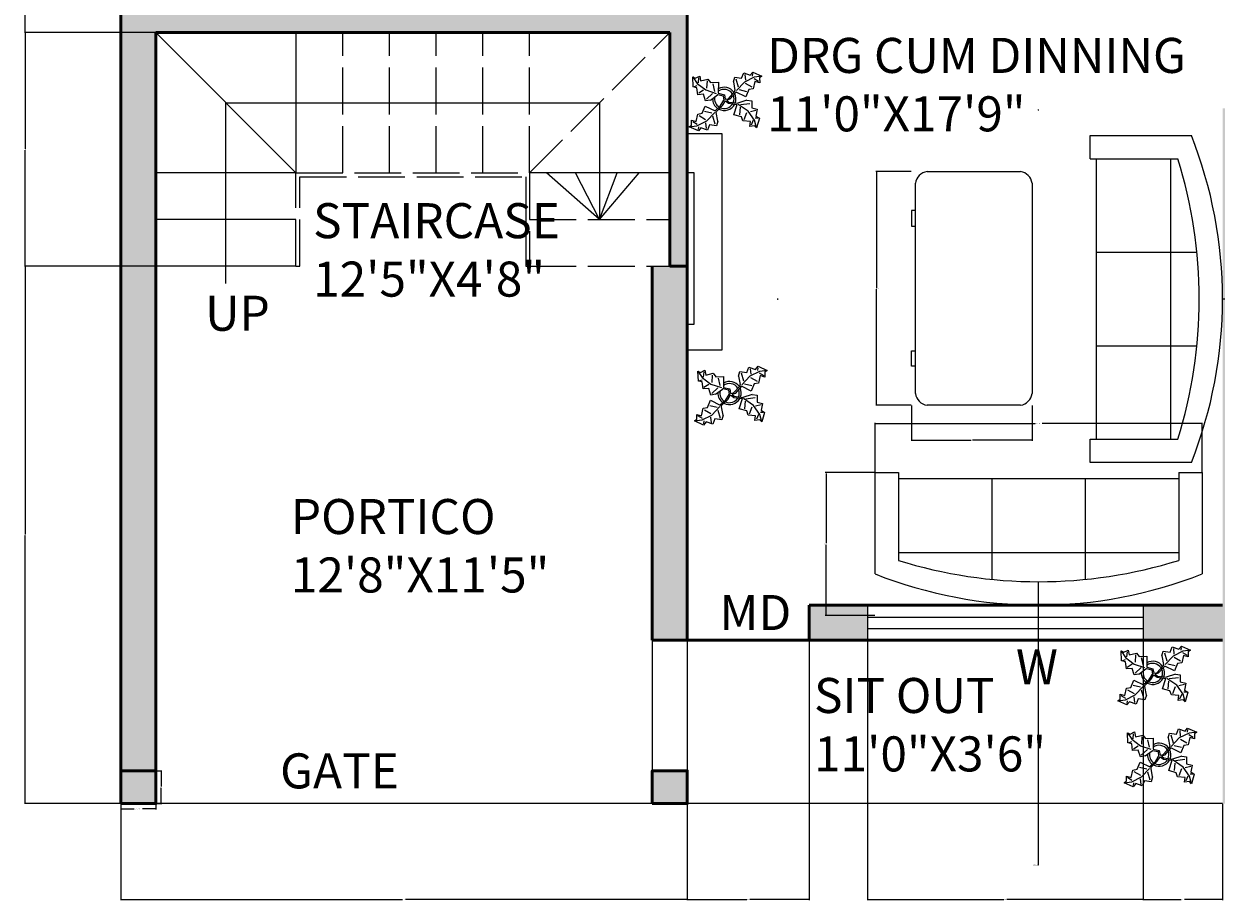
# Model space of a CAD drawing. Units: inches. Extents: x 1099 to 1629, y 1139 to 1548.
# Tile 1 of 3: x 1099 to 1405, y 1139 to 1364. Entities that reach past the tile are written whole.
import ezdxf

# ---------------------------------------------------------------- set-up
doc = ezdxf.new("R2010")
doc.units = ezdxf.units.IN
doc.linetypes.add('ACAD_ISO02W100', pattern=[15, 12, -3])
for name, color, linetype, lineweight in [('A-ANNO-DIMS', 2, 'Continuous', 18), ('A-ANNO-TEXT', 7, 'Continuous', 18), ('A-AREA-IDEN', 7, 'Continuous', 18), ('A-FLOR', 7, 'Continuous', 25), ('A-FLOR-STRS', 7, 'Continuous', 25), ('A-FLOR-STRS-OVHD', 7, 'ACAD_ISO02W100', 18), ('A-FURN', 8, 'Continuous', 20), ('A-FURN-FIXD', 2, 'Continuous', 18), ('A-WALL', 1, 'Continuous', 50), ('L-PLNT', 3, 'Continuous', 18)]:
    doc.layers.add(name, color=color, linetype=linetype, lineweight=lineweight)
for name, color, linetype, lineweight, true_color in [('A-ANNO-SYMB', 244, 'Continuous', 18, 0x991b1e), ('A-COLS', 177, 'Continuous', 50, 0x293189), ('A-GLAZ', 177, 'Continuous', 20, 0x293189), ('A-WALL-PATT', 244, 'Continuous', 13, 0x991b1e)]:
    doc.layers.add(name, color=color, linetype=linetype, lineweight=lineweight, true_color=true_color)
doc.styles.get("Standard").update_dxf_attribs({"font": 'arial.ttf'})
doc.dimstyles.get("Standard").update_dxf_attribs({"dimtxt": 0.18, "dimasz": 0.18, "dimexe": 0.18, "dimexo": 0.0625, "dimgap": 0.09, "dimtad": 0, "dimtih": 1, "dimtoh": 1, "dimdec": 4, "dimzin": 0, "dimdsep": 46, "dimtxsty": 'Standard', "dimcen": 0.09, "dimadec": 0, "dimazin": 0, "dimtfac": 1, "dimtdec": 4, "dimtofl": 0, "dimtmove": 0, "dimatfit": 3, "dimfxl": 1, "dimtolj": 1, "dimtzin": 0, "dimarcsym": 0})

# ---------------------------------------------------------------- blocks, each defined once
blk = doc.blocks.new('Sofa - Roundback 7 ft.')
for p, q in [((-12.00002, -32.4421), (-12.00003, -6.5971)), ((11.99997, -32.4421), (11.99998, -6.5971)), ((-36.000027, -34), (-36.000027, -11.4696)), ((35.99998, -34), (35.99998, -11.4696)), ((-35.999844, -13.3819), (35.9998, -13.3819)), ((-36.000027, -32.4421), (35.99998, -32.4421))]:
    blk.add_line(p, q)
for points in [[(-36.000027, -34), (-42.000027, -34), (-42.000027, -8)], [(41.99998, -8), (41.99998, -34), (35.99998, -34)]]:
    blk.add_lwpolyline(points)
for centre, radius, start, end in [((0, -114.25), 114.25, 68.43141, 111.5686), ((-0.00001, -127.1968), 121.1968, 72.72033, 107.2797)]:
    blk.add_arc(centre, radius, start, end)
blk = doc.blocks.new('Desk - 30 x 60 in.')
for p, q in [((-26.999995, 0), (26.999995, 0)), ((-29.999995, -27), (-29.999995, -3)), ((29.999995, -3), (29.999995, -27)), ((26.999995, -30), (-26.999995, -30)), ((-20.000005, -30), (-20.000005, -31)), ((-16.000005, -31), (-16.000005, -30)), ((15.999995, -31), (15.999995, -30)), ((19.999995, -30), (19.999995, -31)), ((-20.000005, -31), (-16.000005, -31)), ((19.999995, -31), (15.999995, -31))]:
    blk.add_line(p, q)
for centre, start, end in [((-26.499995, -3.5), 98.1301, 171.8699), ((26.499995, -3.5), 8.130102, 81.8699), ((-26.499995, -26.5), 188.1301, 261.8699), ((26.499995, -26.5), 278.1301, 351.8699)]:
    blk.add_arc(centre, 3.535534, start, end)
blk = doc.blocks.new('Plant - Rubber or Philodendron')
for p, q in [((8.8871, 10.7908), (9.9809, 13.4933)), ((9.9809, 13.4933), (13.3837, 12.301)), ((10.5828, 12.6946), (10.8893, 9.7953)), ((13.3837, 12.301), (14.68, 13.9039)), ((14.5816, 13.2037), (14.3848, 11.8033)), ((14.68, 13.9039), (19.3848, 11.8146)), ((-16.2005, 11.4774), (-13.9899, 8.1064)), ((-16.2005, 11.4774), (-14.8639, 10.7964)), ((-16.0159, 6.3329), (-16.2005, 11.4774)), ((-14.0069, 5.8704), (-16.0159, 6.3329)), ((-15.3434, 6.5514), (-13.9984, 6.9884)), ((-14.8639, 10.7964), (-12.6195, 11.8975)), ((-13.9899, 8.1064), (-9.5434, 4.7185)), ((-13.3174, 8.325), (-13.0735, 11.0065)), ((-12.6195, 11.8975), (-12.1909, 9.4345)), ((-12.1909, 9.4345), (-8.3829, 10.3)), ((-8.8369, 9.409), (-9.0894, 5.6095)), ((-8.3829, 10.3), (-7.0549, 8.501)), ((-7.0549, 8.501), (-3.0284, 8.6941)), ((-4.8529, 4.012), (-5.7184, 7.82)), ((-3.0284, 8.6941), (-3.0709, 3.1041)), ((4.6914, 8.8812), (5.3859, 11.2828)), ((4.6914, 8.8812), (5.5014, 4.4831)), ((5.3859, 11.2828), (8.8871, 10.7908)), ((5.9878, 10.4842), (7.1971, 6.3869)), ((10.3916, 8.7942), (6.2847, 4.4028)), ((15.3859, 11.3055), (10.3916, 8.7942)), ((14.2977, 6.1031), (10.9934, 7.9956)), ((15.7909, 9.1065), (14.8995, 5.3044)), ((15.2875, 10.6053), (17.5907, 9.2105)), ((19.3848, 11.8146), (15.3859, 11.3055)), ((18.1925, 8.4119), (15.7909, 9.1065)), ((19.3848, 11.8146), (18.1868, 10.9119)), ((18.1868, 10.9119), (18.1925, 8.4119)), ((-13.5868, 2.2894), (-14.0069, 5.8704)), ((-10.6784, 2.491), (-13.5868, 2.2894)), ((-13.1329, 3.1804), (-10.6614, 4.727)), ((-9.5858, -0.8715), (-10.6784, 2.491)), ((-9.5434, 4.7185), (-4.1917, 2.9888)), ((-9.1318, 0.0195), (-5.9793, 2.9025)), ((-7.1228, -0.443), (-3.5248, 2.2131)), ((-3.5248, 2.2131), (-3.3011, 2.4355)), ((-3.3011, 2.4355), (-0.5306, 1.7947)), ((-3.0709, 3.1041), (0.0797, 2.3163)), ((-0.5306, 1.7947), (-0.2255, -0.5527)), ((-0.5306, 1.7947), (-0.5306, 1.7947)), ((0.0797, 2.3163), (0.4866, -0.031)), ((0.4866, -0.031), (2.1141, 0.2298)), ((2.1141, 0.2298), (5.4346, 3.9146)), ((6.1032, 3.6844), (2.8262, -0.031)), ((5.4346, 3.9146), (5.5014, 4.4831)), ((11.1089, 1.1958), (6.1032, 3.6844)), ((7.7005, 4.8881), (11.5025, 3.9967)), ((12.7005, 4.8994), (11.1089, 1.1958)), ((14.8995, 5.3044), (12.7005, 4.8994)), ((-11.3237, -7.2629), (-9.7321, -3.5593)), ((-9.7321, -3.5593), (-4.7264, -6.0479)), ((-7.1228, -0.443), (-9.5858, -0.8715)), ((-2.019, -3.6148), (-4.7264, -6.0479)), ((-4.0579, -6.2781), (-0.9375, -3.1608)), ((-2.019, -3.6148), (-0.2255, -0.5527)), ((-0.9375, -3.1608), (0.5883, -0.8135)), ((0.5883, -0.8135), (2.2447, -2.0916)), ((2.8262, -0.031), (1.3003, -0.5527)), ((1.3003, -0.5527), (2.4193, -1.4655)), ((2.2447, -2.0916), (6.7108, -2.6626)), ((2.4193, -1.4655), (6.895, -2.1175)), ((4.943, -7.9659), (6.7108, -2.6626)), ((11.6605, -0.5413), (6.895, -2.1175)), ((12.3677, -6.1981), (7.219, -2.6772)), ((8.125, -4.0768), (7.7715, -7.9659)), ((8.3544, -2.7453), (13.1973, -2.1704)), ((11.6605, -0.5413), (14.1354, -0.8948)), ((16.2567, -5.8446), (13.4283, -6.5517)), ((14.1354, -0.8948), (14.1354, -4.4304)), ((14.1354, -4.4304), (16.9638, -5.1375)), ((16.9638, -5.1375), (16.2567, -8.673)), ((-16.8157, -10.7754), (-14.4141, -11.4699)), ((-16.8101, -13.2754), (-16.8157, -10.7754)), ((-13.9107, -12.9688), (-16.2139, -11.574)), ((-14.4141, -11.4699), (-13.5228, -7.6679)), ((-14.0091, -13.669), (-9.0148, -11.1577)), ((-13.5228, -7.6679), (-11.3237, -7.2629)), ((-12.921, -8.4665), (-9.6166, -10.359)), ((-6.3237, -7.2516), (-10.1257, -6.3602)), ((-9.206, -15.0581), (-9.5126, -12.1588)), ((-9.0148, -11.1577), (-4.9047, -6.8122)), ((-4.611, -12.8477), (-5.8203, -8.7504)), ((-4.1246, -6.8466), (-4.0579, -6.2781)), ((-3.3146, -11.2447), (-4.1246, -6.8466)), ((-3.3146, -11.2447), (-4.0092, -13.6463)), ((8.8321, -9.0266), (4.943, -7.9659)), ((9.5392, -11.1479), (8.8321, -9.0266)), ((13.4283, -11.5015), (9.5392, -11.1479)), ((10.2463, -10.4408), (11.6605, -6.9053)), ((15.5496, -10.7943), (12.3677, -6.1981)), ((13.0748, -13.9763), (13.4283, -11.5015)), ((14.8425, -10.7943), (13.7819, -13.2692)), ((16.6103, -14.6834), (15.5496, -10.7943)), ((17.3174, -9.7337), (15.9032, -9.7337)), ((16.2567, -8.673), (18.0245, -9.7337)), ((18.0245, -9.7337), (16.6103, -14.6834)), ((-18.008, -14.1781), (-16.8101, -13.2754)), ((-18.008, -14.1781), (-14.0091, -13.669)), ((-13.3032, -16.2674), (-18.008, -14.1781)), ((-12.0069, -14.6645), (-13.3032, -16.2674)), ((-13.2048, -15.5672), (-13.008, -14.1668)), ((-8.6042, -15.8568), (-12.0069, -14.6645)), ((-7.5103, -13.1543), (-8.6042, -15.8568)), ((-4.0092, -13.6463), (-7.5103, -13.1543)), ((15.5496, -13.6228), (13.0748, -13.9763)), ((16.6103, -14.6834), (15.5496, -13.6228))]:
    blk.add_line(p, q)
for centre, radius, start, end in [((0, 0), 6.1275, 34.37569, 120.1028), ((0.0308, 0.1664), 6, 178.6147, 235.1169), ((0.0308, 0.1664), 5, 168.1647, 238.6725), ((-0.0601, -0.2075), 5.2461, 33.82192, 124.9414), ((-0.2664, 0.1682), 5.2775, 338.4094, 20.03007), ((-0.098, 0.1364), 6.1288, 341.2017, 26.09184), ((-0.0234, 0.3825), 6.1492, 242.5812, 331.2714), ((-0.1102, 0.4886), 5.2883, 247.3711, 327.472)]:
    blk.add_arc(centre, radius, start, end)
blk = doc.blocks.new('COL-RECT-9IN')
h = blk.add_hatch(color=256)
h.dxf.hatch_style = 1
h.paths.add_polyline_path([(9, 8.44), (0, 8.44), (0, 0), (9, 0)])
blk.add_lwpolyline([(0, 0), (9, 0), (9, 8.44), (0, 8.44)], close=True)
blk = doc.blocks.new('*D13')
at = {"layer": 'A-ANNO-DIMS', "color": 0, "lineweight": -2, "transparency": 16777216}
for p, q in [((1317.85, 1248.69), (1317.85, 1261.41)), ((1318.03, 1261.23), (1358.94, 1261.23)), ((1401.67, 1261.23), (1360.75, 1261.23)), ((1401.85, 1248.69), (1401.85, 1261.41))]:
    blk.add_line(p, q, dxfattribs=at)
at = {"layer": 'A-ANNO-DIMS', "color": 0, "lineweight": 100, "transparency": 16777216}
for points in [[(1318.03, 1261.26), (1318.03, 1261.2), (1317.85, 1261.23)], [(1401.67, 1261.26), (1401.67, 1261.2), (1401.85, 1261.23)]]:
    blk.add_solid(points, dxfattribs=at)
at = {"layer": 'Defpoints', "color": 0, "lineweight": 100, "transparency": 16777216}
for p in [(1317.85, 1261.23), (1317.85, 1248.63), (1401.85, 1248.63)]:
    blk.add_point(p, dxfattribs=at)
at = {"layer": 'A-ANNO-DIMS', "color": 0, "transparency": 16777216, "insert": (1359.85, 1261.23), "char_height": 0.18, "attachment_point": 5}
blk.add_mtext('\\A1;SOFA 84 TYP.', dxfattribs=at)
blk = doc.blocks.new('*D14')
at = {"layer": 'A-ANNO-DIMS', "color": 0, "lineweight": -2, "transparency": 16777216}
for p, q in [((1317.79, 1248.63), (1305.07, 1248.63)), ((1305.25, 1248.45), (1305.25, 1230.48)), ((1305.25, 1212.14), (1305.25, 1230.11)), ((1317.79, 1211.96), (1305.07, 1211.96))]:
    blk.add_line(p, q, dxfattribs=at)
at = {"layer": 'A-ANNO-DIMS', "color": 0, "lineweight": 100, "transparency": 16777216}
for points in [[(1305.22, 1248.45), (1305.28, 1248.45), (1305.25, 1248.63)], [(1305.22, 1212.14), (1305.28, 1212.14), (1305.25, 1211.96)]]:
    blk.add_solid(points, dxfattribs=at)
at = {"layer": 'Defpoints', "color": 0, "lineweight": 100, "transparency": 16777216}
for p in [(1317.85, 1248.63), (1305.25, 1211.96), (1317.85, 1211.96)]:
    blk.add_point(p, dxfattribs=at)
at = {"layer": 'A-ANNO-DIMS', "color": 0, "transparency": 16777216, "insert": (1305.25, 1230.29), "char_height": 0.18, "attachment_point": 5}
blk.add_mtext('\\A1;37 TYP.', dxfattribs=at)
blk = doc.blocks.new('*D19')
at = {"layer": 'A-ANNO-DIMS', "color": 0, "lineweight": -2, "transparency": 16777216}
for p, q in [((1327.14, 1325.95), (1318.02, 1325.95)), ((1318.2, 1325.77), (1318.2, 1296.13)), ((1318.2, 1266.13), (1318.2, 1295.77)), ((1327.14, 1265.95), (1318.02, 1265.95))]:
    blk.add_line(p, q, dxfattribs=at)
at = {"layer": 'A-ANNO-DIMS', "color": 0, "lineweight": 100, "transparency": 16777216}
for points in [[(1318.17, 1325.77), (1318.23, 1325.77), (1318.2, 1325.95)], [(1318.17, 1266.13), (1318.23, 1266.13), (1318.2, 1265.95)]]:
    blk.add_solid(points, dxfattribs=at)
at = {"layer": 'Defpoints', "color": 0, "lineweight": 100, "transparency": 16777216}
for p in [(1327.2, 1325.95), (1318.2, 1265.95), (1327.2, 1265.95)]:
    blk.add_point(p, dxfattribs=at)
at = {"layer": 'A-ANNO-DIMS', "color": 0, "transparency": 16777216, "insert": (1318.2, 1295.95), "char_height": 0.18, "attachment_point": 5}
blk.add_mtext('\\A1;DESK 60', dxfattribs=at)
blk = doc.blocks.new('*D20')
at = {"layer": 'A-ANNO-DIMS', "color": 0, "lineweight": -2, "transparency": 16777216}
for p, q in [((1327.2, 1265.89), (1327.2, 1256.77)), ((1358.2, 1265.89), (1358.2, 1256.77)), ((1327.38, 1256.95), (1342.5, 1256.95)), ((1358.02, 1256.95), (1342.91, 1256.95))]:
    blk.add_line(p, q, dxfattribs=at)
at = {"layer": 'A-ANNO-DIMS', "color": 0, "lineweight": 100, "transparency": 16777216}
for points in [[(1327.38, 1256.98), (1327.38, 1256.92), (1327.2, 1256.95)], [(1358.02, 1256.98), (1358.02, 1256.92), (1358.2, 1256.95)]]:
    blk.add_solid(points, dxfattribs=at)
at = {"layer": 'Defpoints', "color": 0, "lineweight": 100, "transparency": 16777216}
for p in [(1327.2, 1265.95), (1358.2, 1265.95), (1358.2, 1256.95)]:
    blk.add_point(p, dxfattribs=at)
at = {"layer": 'A-ANNO-DIMS', "color": 0, "transparency": 16777216, "insert": (1342.7, 1256.95), "char_height": 0.18, "attachment_point": 5}
blk.add_mtext('\\A1;31', dxfattribs=at)
blk = doc.blocks.new('*D21')
at = {"layer": 'A-ANNO-DIMS', "color": 0, "lineweight": -2, "transparency": 16777216}
for p, q in [((1124.1, 1163.57), (1124.1, 1162.1)), ((1124.28, 1162.28), (1127.56, 1162.28)), ((1132.92, 1162.28), (1129.64, 1162.28)), ((1133.1, 1163.57), (1133.1, 1162.1))]:
    blk.add_line(p, q, dxfattribs=at)
at = {"layer": 'A-ANNO-DIMS', "color": 0, "lineweight": 100, "transparency": 16777216}
for points in [[(1124.28, 1162.31), (1124.28, 1162.25), (1124.1, 1162.28)], [(1132.92, 1162.31), (1132.92, 1162.25), (1133.1, 1162.28)]]:
    blk.add_solid(points, dxfattribs=at)
at = {"layer": 'Defpoints', "color": 0, "lineweight": 100, "transparency": 16777216}
for p in [(1124.1, 1163.63), (1133.1, 1163.63), (1133.1, 1162.28)]:
    blk.add_point(p, dxfattribs=at)
at = {"layer": 'A-ANNO-DIMS', "color": 0, "transparency": 16777216, "insert": (1128.6, 1162.28), "char_height": 0.18, "attachment_point": 5}
blk.add_mtext('\\A1;COLUMN 9 TYP.', dxfattribs=at)
blk = doc.blocks.new('*D22')
at = {"layer": 'A-ANNO-DIMS', "color": 0, "lineweight": -2, "transparency": 16777216}
for p, q in [((1133.16, 1172.07), (1134.63, 1172.07)), ((1134.45, 1171.89), (1134.45, 1168.03)), ((1134.45, 1163.81), (1134.45, 1167.67)), ((1133.16, 1163.63), (1134.63, 1163.63))]:
    blk.add_line(p, q, dxfattribs=at)
at = {"layer": 'A-ANNO-DIMS', "color": 0, "lineweight": 100, "transparency": 16777216}
for points in [[(1134.42, 1171.89), (1134.48, 1171.89), (1134.45, 1172.07)], [(1134.42, 1163.81), (1134.48, 1163.81), (1134.45, 1163.63)]]:
    blk.add_solid(points, dxfattribs=at)
at = {"layer": 'Defpoints', "color": 0, "lineweight": 100, "transparency": 16777216}
for p in [(1133.1, 1172.07), (1134.45, 1172.07), (1133.1, 1163.63)]:
    blk.add_point(p, dxfattribs=at)
at = {"layer": 'A-ANNO-DIMS', "color": 0, "transparency": 16777216, "insert": (1134.45, 1167.85), "char_height": 0.18, "attachment_point": 5}
blk.add_mtext('\\A1;8 TYP.', dxfattribs=at)
blk = doc.blocks.new('*D27')
at = {"layer": 'A-ANNO-DIMS', "color": 0, "lineweight": -2, "transparency": 16777216}
for p, q in [((1124.1, 1163.57), (1124.1, 1138.85)), ((1269.6, 1163.57), (1269.6, 1138.85)), ((1124.28, 1139.03), (1196.46, 1139.03)), ((1269.42, 1139.03), (1197.23, 1139.03))]:
    blk.add_line(p, q, dxfattribs=at)
at = {"layer": 'A-ANNO-DIMS', "color": 0, "lineweight": 100, "transparency": 16777216}
for points in [[(1124.28, 1139.06), (1124.28, 1139), (1124.1, 1139.03)], [(1269.42, 1139.06), (1269.42, 1139), (1269.6, 1139.03)]]:
    blk.add_solid(points, dxfattribs=at)
at = {"layer": 'Defpoints', "color": 0, "lineweight": 100, "transparency": 16777216}
for p in [(1124.1, 1163.63), (1269.6, 1163.63), (1269.6, 1139.03)]:
    blk.add_point(p, dxfattribs=at)
at = {"layer": 'A-ANNO-DIMS', "color": 0, "transparency": 16777216, "insert": (1196.85, 1139.03), "char_height": 0.18, "attachment_point": 5}
blk.add_mtext('\\A1;145.5', dxfattribs=at)
blk = doc.blocks.new('*D28')
at = {"layer": 'A-ANNO-DIMS', "color": 0, "lineweight": -2, "transparency": 16777216}
for p, q in [((1269.6, 1205.57), (1269.6, 1138.85)), ((1300.96, 1205.57), (1300.96, 1138.85)), ((1269.78, 1139.03), (1284.88, 1139.03)), ((1300.78, 1139.03), (1285.67, 1139.03))]:
    blk.add_line(p, q, dxfattribs=at)
at = {"layer": 'A-ANNO-DIMS', "color": 0, "lineweight": 100, "transparency": 16777216}
for points in [[(1269.78, 1139.06), (1269.78, 1139), (1269.6, 1139.03)], [(1300.78, 1139.06), (1300.78, 1139), (1300.96, 1139.03)]]:
    blk.add_solid(points, dxfattribs=at)
at = {"layer": 'Defpoints', "color": 0, "lineweight": 100, "transparency": 16777216}
for p in [(1269.6, 1205.63), (1300.96, 1205.63), (1300.96, 1139.03)]:
    blk.add_point(p, dxfattribs=at)
at = {"layer": 'A-ANNO-DIMS', "color": 0, "transparency": 16777216, "insert": (1285.28, 1139.03), "char_height": 0.18, "attachment_point": 5}
blk.add_mtext('\\A1;31.36', dxfattribs=at)
blk = doc.blocks.new('*D29')
at = {"layer": 'A-ANNO-DIMS', "color": 0, "lineweight": -2, "transparency": 16777216}
for p, q in [((1315.91, 1205.57), (1315.91, 1138.85)), ((1386.73, 1205.57), (1386.73, 1138.85)), ((1316.09, 1139.03), (1350.92, 1139.03)), ((1386.55, 1139.03), (1351.71, 1139.03))]:
    blk.add_line(p, q, dxfattribs=at)
at = {"layer": 'A-ANNO-DIMS', "color": 0, "lineweight": 100, "transparency": 16777216}
for points in [[(1316.09, 1139.06), (1316.09, 1139), (1315.91, 1139.03)], [(1386.55, 1139.06), (1386.55, 1139), (1386.73, 1139.03)]]:
    blk.add_solid(points, dxfattribs=at)
at = {"layer": 'Defpoints', "color": 0, "lineweight": 100, "transparency": 16777216}
for p in [(1315.91, 1205.63), (1386.73, 1205.63), (1386.73, 1139.03)]:
    blk.add_point(p, dxfattribs=at)
at = {"layer": 'A-ANNO-DIMS', "color": 0, "transparency": 16777216, "insert": (1351.32, 1139.03), "char_height": 0.18, "attachment_point": 5}
blk.add_mtext('\\A1;70.82', dxfattribs=at)
blk = doc.blocks.new('*D30')
at = {"layer": 'A-ANNO-DIMS', "color": 0, "lineweight": -2, "transparency": 16777216}
for p, q in [((1386.73, 1205.57), (1386.73, 1138.85)), ((1407.1, 1163.57), (1407.1, 1138.85)), ((1386.91, 1139.03), (1396.52, 1139.03)), ((1406.92, 1139.03), (1397.31, 1139.03))]:
    blk.add_line(p, q, dxfattribs=at)
at = {"layer": 'A-ANNO-DIMS', "color": 0, "lineweight": 100, "transparency": 16777216}
for points in [[(1386.91, 1139.06), (1386.91, 1139), (1386.73, 1139.03)], [(1406.92, 1139.06), (1406.92, 1139), (1407.1, 1139.03)]]:
    blk.add_solid(points, dxfattribs=at)
at = {"layer": 'Defpoints', "color": 0, "lineweight": 100, "transparency": 16777216}
for p in [(1386.73, 1205.63), (1407.1, 1163.63), (1407.1, 1139.03)]:
    blk.add_point(p, dxfattribs=at)
at = {"layer": 'A-ANNO-DIMS', "color": 0, "transparency": 16777216, "insert": (1396.91, 1139.03), "char_height": 0.18, "attachment_point": 5}
blk.add_mtext('\\A1;20.37', dxfattribs=at)
blk = doc.blocks.new('*D34')
at = {"layer": 'A-ANNO-DIMS', "color": 0, "lineweight": -2, "transparency": 16777216}
for p, q in [((1133.04, 1301.63), (1099.32, 1301.63)), ((1099.5, 1301.45), (1099.5, 1232.81)), ((1099.5, 1163.81), (1099.5, 1232.45)), ((1124.04, 1163.63), (1099.32, 1163.63))]:
    blk.add_line(p, q, dxfattribs=at)
at = {"layer": 'A-ANNO-DIMS', "color": 0, "lineweight": 100, "transparency": 16777216}
for points in [[(1099.47, 1301.45), (1099.53, 1301.45), (1099.5, 1301.63)], [(1099.47, 1163.81), (1099.53, 1163.81), (1099.5, 1163.63)]]:
    blk.add_solid(points, dxfattribs=at)
at = {"layer": 'Defpoints', "color": 0, "lineweight": 100, "transparency": 16777216}
for p in [(1099.5, 1301.63), (1133.1, 1301.63), (1124.1, 1163.63)]:
    blk.add_point(p, dxfattribs=at)
at = {"layer": 'A-ANNO-DIMS', "color": 0, "transparency": 16777216, "insert": (1099.5, 1232.63), "char_height": 0.18, "attachment_point": 5}
blk.add_mtext('\\A1;138', dxfattribs=at)
blk = doc.blocks.new('*D35')
at = {"layer": 'A-ANNO-DIMS', "color": 0, "lineweight": -2, "transparency": 16777216}
for p, q in [((1133.04, 1361.63), (1099.32, 1361.63)), ((1099.5, 1361.45), (1099.5, 1331.81)), ((1099.5, 1301.81), (1099.5, 1331.45)), ((1133.04, 1301.63), (1099.32, 1301.63))]:
    blk.add_line(p, q, dxfattribs=at)
at = {"layer": 'A-ANNO-DIMS', "color": 0, "lineweight": 100, "transparency": 16777216}
for points in [[(1099.47, 1361.45), (1099.53, 1361.45), (1099.5, 1361.63)], [(1099.47, 1301.81), (1099.53, 1301.81), (1099.5, 1301.63)]]:
    blk.add_solid(points, dxfattribs=at)
at = {"layer": 'Defpoints', "color": 0, "lineweight": 100, "transparency": 16777216}
for p in [(1099.5, 1361.63), (1133.1, 1361.63), (1133.1, 1301.63)]:
    blk.add_point(p, dxfattribs=at)
at = {"layer": 'A-ANNO-DIMS', "color": 0, "transparency": 16777216, "insert": (1099.5, 1331.63), "char_height": 0.18, "attachment_point": 5}
blk.add_mtext('\\A1;60', dxfattribs=at)
blk = doc.blocks.new('*D36')
at = {"layer": 'A-ANNO-DIMS', "color": 0, "lineweight": -2, "transparency": 16777216}
for p, q in [((1133.04, 1462.13), (1099.32, 1462.13)), ((1099.5, 1461.95), (1099.5, 1412.06)), ((1099.5, 1361.81), (1099.5, 1411.7)), ((1133.04, 1361.63), (1099.32, 1361.63))]:
    blk.add_line(p, q, dxfattribs=at)
at = {"layer": 'A-ANNO-DIMS', "color": 0, "lineweight": 100, "transparency": 16777216}
for points in [[(1099.47, 1461.95), (1099.53, 1461.95), (1099.5, 1462.13)], [(1099.47, 1361.81), (1099.53, 1361.81), (1099.5, 1361.63)]]:
    blk.add_solid(points, dxfattribs=at)
at = {"layer": 'Defpoints', "color": 0, "lineweight": 100, "transparency": 16777216}
for p in [(1099.5, 1462.13), (1133.1, 1462.13), (1133.1, 1361.63)]:
    blk.add_point(p, dxfattribs=at)
at = {"layer": 'A-ANNO-DIMS', "color": 0, "transparency": 16777216, "insert": (1099.5, 1411.88), "char_height": 0.18, "attachment_point": 5}
blk.add_mtext('\\A1;100.5', dxfattribs=at)
blk = doc.blocks.new('*D38')
at = {"layer": 'A-ANNO-DIMS', "color": 0, "lineweight": -2, "transparency": 16777216}
for p, q in [((1292.76, 1293.22), (1292.94, 1293.22)), ((1292.85, 1293.13), (1292.85, 1293.31)), ((1475.65, 1293.22), (1407.28, 1293.22))]:
    blk.add_line(p, q, dxfattribs=at)
at = {"layer": 'A-ANNO-DIMS', "color": 0, "lineweight": 100, "transparency": 16777216}
blk.add_solid([(1407.28, 1293.25), (1407.28, 1293.19), (1407.1, 1293.22)], dxfattribs=at)
at = {"layer": 'Defpoints', "color": 0, "lineweight": 100, "transparency": 16777216}
for p in [(1292.85, 1293.22), (1407.1, 1293.22)]:
    blk.add_point(p, dxfattribs=at)
at = {"layer": 'A-ANNO-DIMS', "color": 0, "transparency": 16777216, "insert": (1476.39, 1293.22), "char_height": 0.18, "attachment_point": 5}
blk.add_mtext('\\A1;2X R114.25', dxfattribs=at)
blk = doc.blocks.new('*D39')
at = {"layer": 'A-ANNO-DIMS', "color": 0, "lineweight": -2, "transparency": 16777216}
for p, q in [((1359.76, 1341.82), (1359.94, 1341.82)), ((1359.85, 1341.73), (1359.85, 1341.91)), ((1359.85, 1147.91), (1359.85, 1220.45)), ((1359.67, 1147.91), (1359.85, 1147.91))]:
    blk.add_line(p, q, dxfattribs=at)
at = {"layer": 'A-ANNO-DIMS', "color": 0, "lineweight": 100, "transparency": 16777216}
blk.add_solid([(1359.82, 1220.45), (1359.88, 1220.45), (1359.85, 1220.63)], dxfattribs=at)
at = {"layer": 'Defpoints', "color": 0, "lineweight": 100, "transparency": 16777216}
for p in [(1359.85, 1341.82), (1359.85, 1220.63)]:
    blk.add_point(p, dxfattribs=at)
at = {"layer": 'A-ANNO-DIMS', "color": 0, "transparency": 16777216, "insert": (1358.99, 1147.91), "char_height": 0.18, "attachment_point": 5}
blk.add_mtext('\\A1;2X R121.2', dxfattribs=at)

msp = doc.modelspace()

# ---------------------------------------------------------------- hatches: boundary and pattern name
at = {"layer": 'A-WALL-PATT'}
h = msp.add_hatch(color=256, dxfattribs=at)
h.dxf.hatch_style = 1
h.paths.add_polyline_path([(1407.099, 1523.072), (1416.099, 1523.072), (1416.099, 1514.628), (1595.099, 1514.628), (1595.099, 1523.072), (1604.099, 1523.072), (1604.099, 1523.628), (1124.099, 1523.628), (1124.099, 1172.072), (1133.099, 1172.072), (1133.099, 1361.628), (1265.099, 1361.628), (1265.099, 1301.628), (1269.599, 1301.628), (1269.599, 1366.128), (1133.099, 1366.128), (1133.099, 1462.128), (1169.127, 1462.128), (1169.127, 1466.628), (1133.099, 1466.628), (1133.099, 1514.628), (1265.099, 1514.628), (1265.099, 1514.872), (1265.099, 1523.316), (1274.099, 1523.316), (1274.099, 1514.628), (1326.599, 1514.628), (1326.599, 1508.465), (1331.099, 1508.465), (1331.099, 1514.628), (1407.099, 1514.628)])
h.paths.add_polyline_path([(1604.099, 1514.628), (1595.099, 1514.628), (1595.099, 1384.628), (1595.099, 1380.128), (1595.099, 1323.878), (1535.099, 1323.878), (1535.099, 1321.628), (1595.099, 1321.628), (1595.099, 1172.628), (1539.988, 1172.628), (1539.988, 1163.628), (1594.904, 1163.628), (1594.904, 1172.072), (1604.099, 1172.072)])
h.paths.add_polyline_path([(1461.599, 1380.128), (1530.599, 1380.128), (1530.599, 1363.564), (1535.099, 1363.564), (1535.099, 1380.128), (1535.099, 1384.628), (1416.099, 1384.628), (1416.099, 1380.128), (1457.099, 1380.128), (1457.099, 1326.128), (1457.099, 1321.628), (1504.951, 1321.628), (1504.951, 1326.128), (1461.599, 1326.128)], flags=17)
h.paths.add_polyline_path([(1535.099, 1346.252), (1530.599, 1346.252), (1530.599, 1326.128), (1530.599, 1321.628), (1535.099, 1321.628), (1535.099, 1323.878), (1535.099, 1326.128)], flags=16)
h.paths.add_polyline_path([(1269.599, 1301.628), (1265.099, 1301.628), (1260.599, 1301.628), (1260.599, 1214.628), (1260.599, 1205.628), (1265.099, 1205.628), (1269.599, 1205.628), (1269.599, 1214.628)], flags=17)
h.paths.add_polyline_path([(1411.599, 1262.279), (1451.001, 1262.279), (1451.001, 1266.779), (1411.599, 1266.779), (1411.599, 1342.184), (1407.099, 1342.184), (1407.099, 1214.628), (1386.727, 1214.628), (1386.727, 1205.628), (1407.099, 1205.628), (1407.099, 1163.628), (1491.988, 1163.628), (1491.988, 1172.628), (1411.599, 1172.628)])
h.paths.add_polyline_path([(1315.906, 1214.628), (1300.958, 1214.628), (1300.958, 1205.628), (1315.906, 1205.628)], flags=17)

# ---------------------------------------------------------------- linework, layer by layer
at = {"layer": 'A-ANNO-SYMB'}
for p, q in [((1151.099, 1297.207), (1151.099, 1343.628)), ((1151.099, 1343.628), (1247.099, 1343.628)), ((1247.099, 1343.628), (1247.099, 1313.628)), ((1247.099, 1313.628), (1233.474, 1325.628)), ((1247.099, 1313.628), (1240.927, 1325.628)), ((1247.099, 1313.628), (1251.56, 1325.628)), ((1247.099, 1313.628), (1257.227, 1325.628))]:
    msp.add_line(p, q, dxfattribs=at)
at = {"layer": 'A-FLOR'}
for p, q in [((1260.599, 1205.628), (1260.599, 1163.628)), ((1407.099, 1163.628), (1133.099, 1163.628))]:
    msp.add_line(p, q, dxfattribs=at)
at = {"layer": 'A-FLOR-STRS'}
for p, q in [((1169.099, 1325.628), (1133.099, 1361.628)), ((1169.099, 1361.628), (1169.099, 1325.628)), ((1169.099, 1325.628), (1133.099, 1325.628)), ((1265.099, 1325.628), (1229.099, 1325.628)), ((1169.099, 1313.628), (1133.099, 1313.628)), ((1169.099, 1301.628), (1133.099, 1301.628))]:
    msp.add_line(p, q, dxfattribs=at)
at = {"layer": 'A-FLOR-STRS-OVHD'}
for p, q in [((1181.099, 1325.628), (1181.099, 1361.628)), ((1193.099, 1325.628), (1193.099, 1361.628)), ((1205.099, 1325.628), (1205.099, 1361.628)), ((1217.099, 1325.628), (1217.099, 1361.628)), ((1229.099, 1325.628), (1229.099, 1361.628)), ((1229.099, 1325.628), (1265.099, 1361.628)), ((1169.099, 1301.628), (1169.099, 1325.628)), ((1169.099, 1325.628), (1229.099, 1325.628)), ((1170.099, 1301.628), (1170.099, 1324.628)), ((1170.099, 1324.628), (1228.099, 1324.628)), ((1228.099, 1324.628), (1228.099, 1301.628)), ((1229.099, 1325.628), (1229.099, 1301.628)), ((1229.099, 1313.628), (1265.099, 1313.628)), ((1169.099, 1301.628), (1170.099, 1301.628)), ((1228.099, 1301.628), (1229.099, 1301.628)), ((1229.099, 1301.628), (1265.099, 1301.628))]:
    msp.add_line(p, q, dxfattribs=at)
at = {"layer": 'A-FURN-FIXD'}
for p, q in [((1269.599, 1335.703), (1278.483, 1335.703)), ((1278.483, 1335.703), (1278.483, 1280.109)), ((1269.599, 1325.746), (1271.283, 1325.746)), ((1271.283, 1325.746), (1271.283, 1286.677)), ((1271.283, 1286.677), (1269.599, 1286.677)), ((1278.483, 1280.109), (1269.599, 1280.109))]:
    msp.add_line(p, q, dxfattribs=at)
at = {"layer": 'A-GLAZ'}
for p, q in [((1315.906, 1214.628), (1315.906, 1205.628)), ((1386.727, 1214.628), (1386.727, 1205.628)), ((1386.727, 1211.421), (1315.906, 1211.421)), ((1386.727, 1208.493), (1315.906, 1208.493))]:
    msp.add_line(p, q, dxfattribs=at)
at = {"layer": 'A-WALL'}
for p, q in [((1124.099, 1523.628), (1124.099, 1163.628)), ((1269.599, 1366.128), (1269.599, 1301.628)), ((1265.099, 1361.628), (1133.099, 1361.628)), ((1133.099, 1361.628), (1133.099, 1163.628)), ((1265.099, 1361.628), (1265.099, 1301.628)), ((1260.599, 1301.628), (1260.599, 1214.628)), ((1265.099, 1301.628), (1269.599, 1301.628)), ((1269.599, 1301.628), (1269.599, 1214.628)), ((1260.599, 1214.628), (1260.599, 1205.628)), ((1269.599, 1214.628), (1269.599, 1205.628)), ((1300.958, 1214.628), (1300.958, 1205.628)), ((1300.958, 1214.628), (1407.099, 1214.628)), ((1260.599, 1205.628), (1265.099, 1205.628)), ((1265.099, 1205.628), (1407.099, 1205.628)), ((1124.099, 1163.628), (1133.099, 1163.628))]:
    msp.add_line(p, q, dxfattribs=at)

# ---------------------------------------------------------------- block references
at = {"layer": 'A-COLS'}
for p in [(1124.099, 1163.628), (1260.599, 1163.628)]:
    msp.add_blockref('COL-RECT-9IN', p, dxfattribs=at)
at = {"layer": 'A-FURN'}
for name, p, rotation in [('Sofa - Roundback 7 ft.', (1407.099, 1293.22), 270), ('Desk - 30 x 60 in.', (1358.204, 1295.948), 270), ('Sofa - Roundback 7 ft.', (1359.848, 1214.628), 179.9999778310002)]:
    msp.add_blockref(name, p, dxfattribs=dict(at, rotation=rotation))
at = {"layer": 'L-PLNT', "xscale": 0.5, "yscale": 0.5}
for p in [(1279.11, 1344.534), (1280.461, 1268.983), (1389.191, 1197.128), (1390.804, 1176.095)]:
    msp.add_blockref('Plant - Rubber or Philodendron', p, dxfattribs=at)

# ---------------------------------------------------------------- texts
at = {"layer": 'A-ANNO-TEXT', "char_height": 9, "attachment_point": 1}
for s, width, insert in [('UP', 16.11456, (1145.75, 1294.061)), ('MD', 16.11456, (1277.902, 1217.207)), ('W', 16.11456, (1354.039, 1203.249)), ('GATE', 77.99839, (1165.015, 1176.542))]:
    msp.add_mtext_dynamic_manual_height_columns(s, width=width, gutter_width=12.5, heights=[0], dxfattribs=dict(at, insert=insert))
at = {"layer": 'A-AREA-IDEN', "char_height": 9, "attachment_point": 1}
for s, width, insert in [('DRG CUM DINNING\\P11\'0"X17\'9"', 138.29385, (1290.111, 1360.273)), ('STAIRCASE\\P12\'5"X4\'8"', 79.89808, (1173.495, 1317.834)), ('PORTICO\\P12\'8"X11\'5"', 79.89808, (1167.776, 1241.854)), ('SIT OUT\\P11\'0"X3\'6"', 79.89808, (1302.178, 1195.904))]:
    msp.add_mtext_dynamic_manual_height_columns(s, width=width, gutter_width=12.5, heights=[0], dxfattribs=dict(at, insert=insert))

# ---------------------------------------------------------------- dimensions: what is measured, and where the dimension line sits
at = {"layer": 'A-ANNO-DIMS'}
for base, p1, p2, override, picture, middle in [((1099.499, 1462.128), (1133.099, 1361.628), (1133.099, 1462.128), {"dimdec": 1, "dimlfac": 1, "dimrnd": 0, "dimzin": 0, "dimdsep": 46, "dimlunit": 2}, '*D36', (1099.499, 1411.878)), ((1099.499, 1361.628), (1133.099, 1301.628), (1133.099, 1361.628), {"dimdec": 0, "dimlfac": 1, "dimrnd": 0, "dimzin": 0, "dimdsep": 46, "dimlunit": 2}, '*D35', (1099.499, 1331.628)), ((1099.499, 1301.628), (1124.099, 1163.628), (1133.099, 1301.628), {"dimdec": 0, "dimlfac": 1, "dimrnd": 0, "dimzin": 0, "dimdsep": 46, "dimlunit": 2}, '*D34', (1099.499, 1232.628))]:
    dim = msp.add_linear_dim(base=base, p1=p1, p2=p2, angle=90, dimstyle='Standard', override=override, dxfattribs=at)
    dim.commit()
    dim.dimension.update_dxf_attribs({"geometry": picture, "text_midpoint": middle})
for center, mpoint, override, picture, middle in [((1359.848, 1341.825), (1359.848, 1220.628), {"dimdec": 1, "dimlfac": 1, "dimrnd": 0, "dimzin": 0, "dimdsep": 46, "dimlunit": 2}, '*D39', (1358.994, 1147.91)), ((1292.849, 1293.22), (1407.099, 1293.22), {"dimdec": 2, "dimlfac": 1, "dimrnd": 0, "dimzin": 0, "dimdsep": 46, "dimlunit": 2}, '*D38', (1475.649, 1293.22))]:
    dim = msp.add_radius_dim(center=center, mpoint=mpoint, text='2X <>', dimstyle='Standard', override=override, dxfattribs=at)
    dim.commit()
    dim.dimension.update_dxf_attribs({"geometry": picture, "text_midpoint": middle, "dimtype": 164})
for base, p1, p2, angle, text, picture, middle in [((1318.204, 1265.948), (1327.204, 1325.948), (1327.204, 1265.948), 270, 'DESK <>', '*D19', (1318.204, 1295.948)), ((1317.848, 1261.228), (1401.848, 1248.628), (1317.848, 1248.628), 179.99998, 'SOFA <> TYP.', '*D13', (1359.848, 1261.228)), ((1305.248, 1211.961), (1317.848, 1248.628), (1317.848, 1211.961), 269.99998, '<> TYP.', '*D14', (1305.248, 1230.295)), ((1134.449, 1172.072), (1133.099, 1163.628), (1133.099, 1172.072), 90, '<> TYP.', '*D22', (1134.449, 1167.85))]:
    dim = msp.add_linear_dim(base=base, p1=p1, p2=p2, angle=angle, text=text, dimstyle='Standard', override={"dimdec": 0, "dimlfac": 1, "dimrnd": 0, "dimzin": 0, "dimdsep": 46, "dimlunit": 2}, dxfattribs=at)
    dim.commit()
    dim.dimension.update_dxf_attribs({"geometry": picture, "text_midpoint": middle})
for base, p1, p2, override, picture, middle in [((1358.204, 1256.948), (1327.204, 1265.948), (1358.204, 1265.948), {"dimdec": 0, "dimlfac": 1, "dimrnd": 0, "dimzin": 0, "dimdsep": 46, "dimlunit": 2}, '*D20', (1342.704, 1256.948)), ((1300.958, 1139.028), (1269.599, 1205.628), (1300.958, 1205.628), {"dimdec": 2, "dimlfac": 1, "dimrnd": 0, "dimzin": 0, "dimdsep": 46, "dimlunit": 2}, '*D28', (1285.279, 1139.028)), ((1386.727, 1139.028), (1315.906, 1205.628), (1386.727, 1205.628), {"dimdec": 2, "dimlfac": 1, "dimrnd": 0, "dimzin": 0, "dimdsep": 46, "dimlunit": 2}, '*D29', (1351.317, 1139.028)), ((1407.099, 1139.028), (1386.727, 1205.628), (1407.099, 1163.628), {"dimdec": 2, "dimlfac": 1, "dimrnd": 0, "dimzin": 0, "dimdsep": 46, "dimlunit": 2}, '*D30', (1396.913, 1139.028)), ((1269.599, 1139.028), (1124.099, 1163.628), (1269.599, 1163.628), {"dimdec": 1, "dimlfac": 1, "dimrnd": 0, "dimzin": 0, "dimdsep": 46, "dimlunit": 2}, '*D27', (1196.849, 1139.028))]:
    dim = msp.add_linear_dim(base=base, p1=p1, p2=p2, dimstyle='Standard', override=override, dxfattribs=at)
    dim.commit()
    dim.dimension.update_dxf_attribs({"geometry": picture, "text_midpoint": middle})
dim = msp.add_linear_dim(base=(1133.099, 1162.278), p1=(1124.099, 1163.628), p2=(1133.099, 1163.628), text='COLUMN <> TYP.', dimstyle='Standard', override={"dimdec": 0, "dimlfac": 1, "dimrnd": 0, "dimzin": 0, "dimdsep": 46, "dimlunit": 2}, dxfattribs=at)
dim.commit()
dim.dimension.update_dxf_attribs({"geometry": '*D21', "text_midpoint": (1128.599, 1162.278)})

doc.saveas('drawing.dxf')
